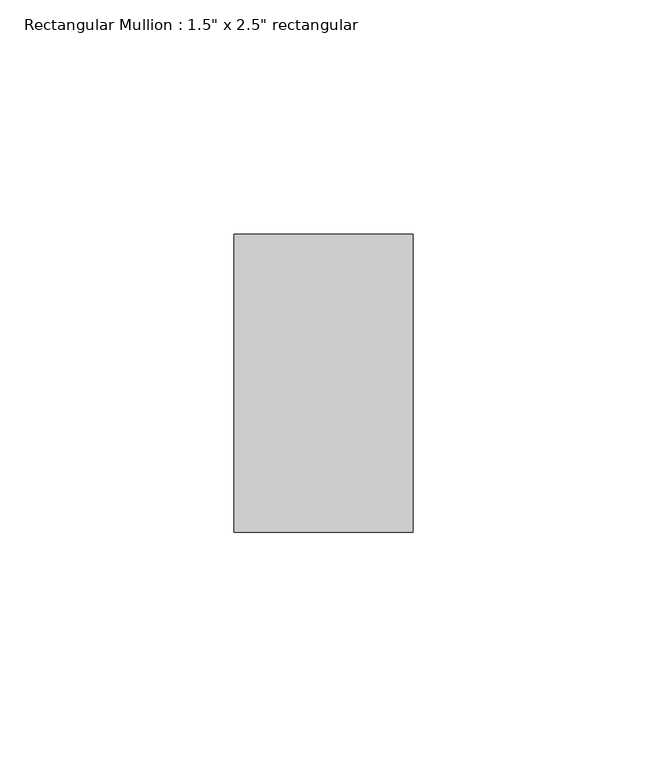
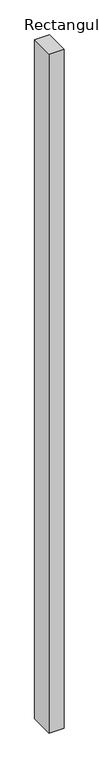
"""IFC4 building model written with IfcOpenShell, lengths in millimetres: member geometry."""

from ifc_helpers import new_model, si_unit, frame, origin, place, context, project, spatial, polyline, outline, extrude, source, transform, mapped, element, save


def member_5c57b440(model_context):
    return source(origin(), model_context, "Body", "SweptSolid", [
        extrude(outline(polyline([(19.05, 31.75), (19.05, -31.75), (-19.05, -31.75), (-19.05, 31.75), (19.05, 31.75)])), frame((0.0, 0.0, -1828.8), z_axis=(0.0, 0.0, 1.0), x_axis=(1.0, 0.0, 0.0)), (0.0, 0.0, 1.0), 1828.8),
    ])


if __name__ == "__main__":
    model = new_model("IFC4")
    model_context = context("Model", 3, world=origin())
    ifc_project = project(units=[si_unit("LENGTHUNIT", "METRE", prefix="MILLI")], contexts=[model_context])
    site = spatial("IfcSite", under=ifc_project)
    building = spatial("IfcBuilding", under=site)
    placement = place(None, origin())
    member_shape = member_5c57b440(model_context)
    element("IfcMember", 1, ObjectType="Rectangular Mullion : 1.5\" x 2.5\" rectangular", at=placement, inside=building, context=model_context, shape_type="MappedRepresentation", body=[
        mapped(member_shape, transform((0.0, 0.0, 0.0), x_axis=(1.0, 0.0, 0.0), y_axis=(0.0, 1.0, 0.0), z_axis=(0.0, 0.0, 1.0))),
    ])
    save(model, "model.ifc")

# Revit data of these elements
# Type "Rectangular Mullion : 1.5\" x 2.5\" rectangular"
#   built-in parameter 1007304 = 0.208333 (stored number, unit not read)
#   built-in parameter 1007301 = 0.0625 (stored number, unit not read)
#   built-in parameter 1007300 = 0.0625 (stored number, unit not read)
# Element 1 (IfcMember, "Rectangular Mullion : 1.5\" x 2.5\" rectangular")
#   Materials on its faces: "Aluminum"
# Materials
#   "Aluminum": class "Metal", colour RGB 247 247 247, transparency 0, Description = "Aluminum 6061", Cost = 0
